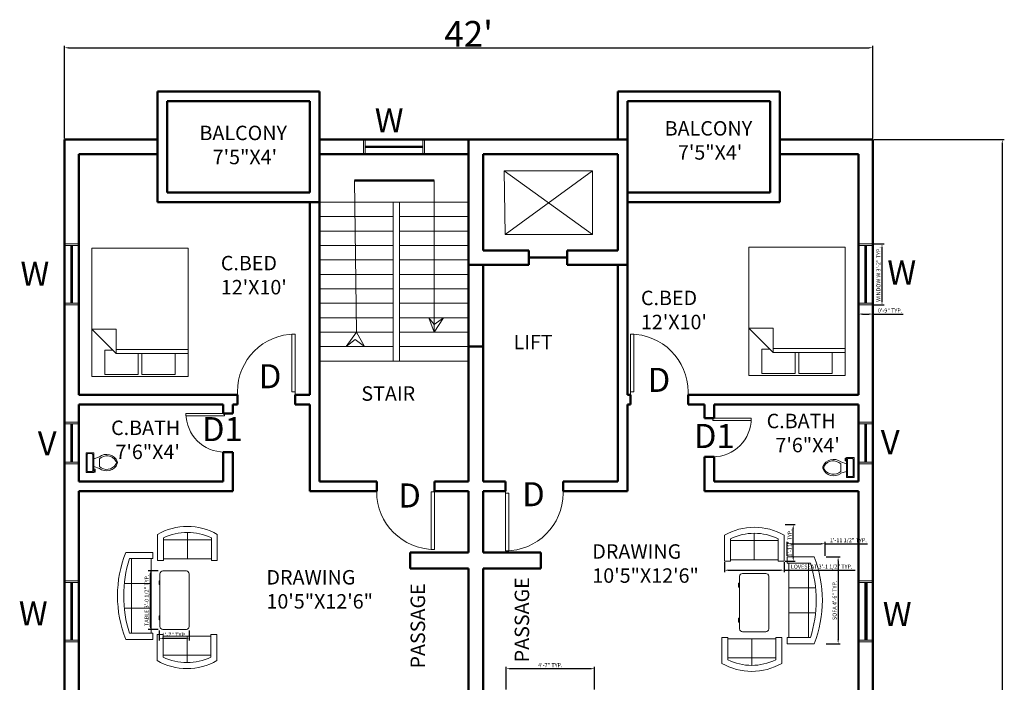
# Model space of a CAD drawing. Units: inches. Extents: x -7040 to -4088, y 6092 to 7645.
# Tile 11 of 11: x -4702 to -4088, y 7176 to 7588. Entities that reach past the tile are written whole.
import ezdxf

# ---------------------------------------------------------------- set-up
doc = ezdxf.new("R2010")
doc.units = ezdxf.units.IN
for name, color, linetype, lineweight in [('A-ANNO-DIMS', 2, 'Continuous', 18), ('A-ANNO-TEXT', 7, 'Continuous', 25), ('A-AREA-IDEN', 3, 'Continuous', 25), ('A-DOOR', 3, 'Continuous', 18), ('A-EQPM', 8, 'Continuous', 18), ('A-FLOR-FIXT', 9, 'Continuous', 13), ('A-FLOR-STRS', 2, 'Continuous', 18), ('A-FURN', 8, 'Continuous', 13), ('A-GLAZ', 4, 'Continuous', 18), ('A-WALL', 7, 'Continuous', 50)]:
    doc.layers.add(name, color=color, linetype=linetype, lineweight=lineweight)
doc.styles.get("Standard").update_dxf_attribs({"font": 'arial.ttf'})
doc.dimstyles.new('ISO-25', dxfattribs={"dimtxt": 2.5, "dimasz": 2.5, "dimexe": 1.25, "dimexo": 0.625, "dimtad": 1, "dimdec": 0, "dimlunit": 3, "dimtxsty": 'Standard', "dimcen": 2.5, "dimadec": 0, "dimazin": 0, "dimtfac": 1, "dimtdec": 0, "dimtmove": 0, "dimatfit": 3, "dimfxl": 1, "dimarcsym": 0})

# ---------------------------------------------------------------- blocks, each defined once
blk = doc.blocks.new('*U8')
for p, q in [((0, 0), (0, -100)), ((750, 0), (750, -100))]:
    blk.add_line(p, q)
blk.add_lwpolyline([(0, 0), (0, 750), (43.75, 750), (43.75, 0)], close=True)
blk.add_arc((0, 0), 750, 0, 90)
blk = doc.blocks.new('Bed - Queen')
for p, q in [((0, -80.00003), (0, 0)), ((0, 0), (59.99999, 0)), ((59.99999, 0), (59.99999, -80.00003)), ((7.99999, -1.2), (28.79998, -1.2)), ((7.99999, -14.4), (7.99999, -1.2)), ((28.79998, -1.2), (28.79998, -14.4)), ((31.19999, -1.2), (51.99999, -1.2)), ((31.19999, -14.4), (31.19999, -1.2)), ((51.99999, -1.2), (51.99999, -16.4)), ((0, -14.4), (44.8, -14.4)), ((44.8, -16.8), (0, -16.8)), ((59.99999, -29.6), (44.8, -14.4)), ((44.8, -14.4), (44.8, -29.6)), ((51.99999, -16.4), (46.79936, -16.4)), ((44.8, -29.6), (59.99999, -29.6)), ((59.99999, -80.00003), (0, -80.00003))]:
    blk.add_line(p, q)
blk = doc.blocks.new('Toilet - top')
for p, q in [((-10, -8.5), (-8, -8.5)), ((-10, -9.5), (-10, -8.5)), ((-7, -9.5), (-10, -9.5)), ((-8, -8.5), (-8, -8)), ((-7, -8), (-7, -9.5)), ((-4, -8), (-6, -14)), ((4, -8), (6, -14)), ((9.5, -6), (9.5, -2)), ((4, -14), (-4, -14))]:
    blk.add_line(p, q)
blk.add_lwpolyline([(10.5, -8), (10.5, 0), (-10.5, 0), (-10.5, -8)], close=True)
for points in [[(-9.5, -2), (-9.5, -6)], [(8.5, -1), (-8.5, -1)], [(-8.5, -7), (8.5, -7)]]:
    blk.add_lwpolyline(points)
for centre, radius, start, end in [((-8.6, -1.9), 0.884, 81.8699, 188.1301), ((-8.6, -6.1), 0.884, 171.8699, 278.1301), ((8.6, -1.9), 0.884, 351.8699, 98.1301), ((8.6, -6.1), 0.884, 261.8699, 8.1301), ((3.5, -21.6), 12.2, 141.4691, 247.9714), ((4.2, -21.8), 11.3, 136.3677, 238.9468), ((-3.5, -21.6), 12.2, 292.0284, 38.5307), ((-4.2, -21.8), 11.3, 301.053, 43.6321), ((0, -27.9), 4, 245.7318, 294.2682), ((0, -29), 4, 254.8605, 285.1395)]:
    blk.add_arc(centre, radius, start, end)
blk = doc.blocks.new('Desk - 30 x 60 in.')
for p, q in [((-26.999995, 0), (26.999995, 0)), ((-29.999995, -27), (-29.999995, -3)), ((29.999995, -3), (29.999995, -27)), ((26.999995, -30), (-26.999995, -30)), ((-20.000005, -30), (-20.000005, -31)), ((-16.000005, -31), (-16.000005, -30)), ((15.999995, -31), (15.999995, -30)), ((19.999995, -30), (19.999995, -31)), ((-20.000005, -31), (-16.000005, -31)), ((19.999995, -31), (15.999995, -31))]:
    blk.add_line(p, q)
for centre, start, end in [((-26.499995, -3.5), 98.1301, 171.8699), ((26.499995, -3.5), 8.130102, 81.8699), ((-26.499995, -26.5), 188.1301, 261.8699), ((26.499995, -26.5), 278.1301, 351.8699)]:
    blk.add_arc(centre, 3.535534, start, end)
blk = doc.blocks.new('Sofa - Roundback 7 ft.')
for p, q in [((-12.00002, -32.4421), (-12.00003, -6.5971)), ((11.99997, -32.4421), (11.99998, -6.5971)), ((-36.000027, -34), (-36.000027, -11.4696)), ((-35.999844, -13.3819), (35.9998, -13.3819)), ((35.99998, -34), (35.99998, -11.4696)), ((-36.000027, -32.4421), (35.99998, -32.4421))]:
    blk.add_line(p, q)
for points in [[(-36.000027, -34), (-42.000027, -34), (-42.000027, -8)], [(41.99998, -8), (41.99998, -34), (35.99998, -34)]]:
    blk.add_lwpolyline(points)
for centre, radius, start, end in [((0, -114.25), 114.25, 68.43141, 111.5686), ((-0.00001, -127.1968), 121.1968, 72.72033, 107.2797)]:
    blk.add_arc(centre, radius, start, end)
blk = doc.blocks.new('Sofa - Roundback Loveseat 5 ft.')
for p, q in [((0, -32.44198), (0, -5.99998)), ((-24, -33.99998), (-24, -11.46958)), ((-23.9998, -13.38178), (23.99986, -13.38178)), ((24.00004, -33.99998), (24.00004, -11.46958)), ((-24, -32.44198), (24.00004, -32.44198))]:
    blk.add_line(p, q)
for points in [[(-24, -33.99998), (-30, -33.99998), (-30, -7.99998)], [(30.00004, -7.99998), (30.00004, -33.99998), (24.00004, -33.99998)]]:
    blk.add_lwpolyline(points)
for centre, radius, start, end in [((0, -60.24998), 60.24998, 60.13715, 119.8628), ((0, -61.38438), 55.38444, 64.32083, 115.6792)]:
    blk.add_arc(centre, radius, start, end)
blk = doc.blocks.new('*D108')
at = {"layer": 'A-ANNO-DIMS', "color": 0, "lineweight": -2, "transparency": 16777216}
for p, q in [((-4673.77, 7514.38), (-4673.77, 7572.26)), ((-4671.27, 7571.01), (-4172.27, 7571.01)), ((-4169.77, 7514.38), (-4169.77, 7572.26))]:
    blk.add_line(p, q, dxfattribs=at)
at = {"layer": 'A-ANNO-DIMS', "color": 0, "transparency": 16777216}
for points in [[(-4671.27, 7571.43), (-4671.27, 7570.59), (-4673.77, 7571.01)], [(-4172.27, 7571.43), (-4172.27, 7570.59), (-4169.77, 7571.01)]]:
    blk.add_solid(points, dxfattribs=at)
at = {"layer": 'Defpoints', "color": 0, "transparency": 16777216}
for p in [(-4169.77, 7571.01), (-4673.77, 7513.76), (-4169.77, 7513.76)]:
    blk.add_point(p, dxfattribs=at)
at = {"layer": 'A-ANNO-DIMS', "color": 0, "transparency": 16777216, "insert": (-4421.77, 7579.67), "char_height": 2.5, "attachment_point": 5}
blk.add_mtext("{\\H6.4x;42'}", dxfattribs=at)
blk = doc.blocks.new('*D109')
at = {"layer": 'A-ANNO-DIMS', "color": 0, "lineweight": -2, "transparency": 16777216}
for p, q in [((-4169.15, 7513.76), (-4087.83, 7513.76)), ((-4089.08, 7511.26), (-4089.08, 6766.26)), ((-4169.15, 6763.76), (-4087.83, 6763.76))]:
    blk.add_line(p, q, dxfattribs=at)
at = {"layer": 'A-ANNO-DIMS', "color": 0, "transparency": 16777216}
for points in [[(-4089.49, 7511.26), (-4088.66, 7511.26), (-4089.08, 7513.76)], [(-4089.49, 6766.26), (-4088.66, 6766.26), (-4089.08, 6763.76)]]:
    blk.add_solid(points, dxfattribs=at)
at = {"layer": 'Defpoints', "color": 0, "transparency": 16777216}
for p in [(-4169.77, 7513.76), (-4169.77, 6763.76), (-4089.08, 6763.76)]:
    blk.add_point(p, dxfattribs=at)
at = {"layer": 'A-ANNO-DIMS', "color": 0, "transparency": 16777216, "insert": (-4097.87, 7138.76), "char_height": 2.5, "attachment_point": 5, "rotation": 90}
blk.add_mtext('{\\H6.4x;62\'-6"}', dxfattribs=at)
blk = doc.blocks.new('WIN-36-B')
for p, q in [((0, 38), (9, 38)), ((0, 37), (9, 37)), ((4, 1), (4, 37)), ((4.5, 1), (4.5, 37)), ((5, 1), (5, 37)), ((0, 1), (9, 1)), ((0, 0), (9, 0))]:
    blk.add_line(p, q)
blk = doc.blocks.new('WIN-24-B')
for p, q in [((0, 26), (9, 26)), ((0, 25), (9, 25)), ((4, 1), (4, 25)), ((4.5, 1), (4.5, 25)), ((5, 1), (5, 25)), ((0, 1), (9, 1)), ((0, 0), (9, 0))]:
    blk.add_line(p, q)
blk = doc.blocks.new('*D118')
at = {"layer": 'A-ANNO-DIMS', "color": 0, "lineweight": -2, "transparency": 16777216}
for p, q in [((-4169.15, 7448.76), (-4162.82, 7448.76)), ((-4164.07, 7413.26), (-4164.07, 7446.26)), ((-4169.15, 7410.76), (-4162.82, 7410.76))]:
    blk.add_line(p, q, dxfattribs=at)
at = {"layer": 'A-ANNO-DIMS', "color": 0, "transparency": 16777216}
for points in [[(-4164.49, 7446.26), (-4163.66, 7446.26), (-4164.07, 7448.76)], [(-4164.49, 7413.26), (-4163.66, 7413.26), (-4164.07, 7410.76)]]:
    blk.add_solid(points, dxfattribs=at)
at = {"layer": 'Defpoints', "color": 0, "transparency": 16777216}
for p in [(-4169.77, 7448.76), (-4164.07, 7448.76), (-4169.77, 7410.76)]:
    blk.add_point(p, dxfattribs=at)
at = {"layer": 'A-ANNO-DIMS', "color": 0, "transparency": 16777216, "insert": (-4165.99, 7429.76), "char_height": 2.5, "attachment_point": 5, "rotation": 90}
blk.add_mtext('WINDOW W 3\'-2" TYP.', dxfattribs=at)
blk = doc.blocks.new('*D119')
at = {"layer": 'A-ANNO-DIMS', "color": 0, "lineweight": -2, "transparency": 16777216}
for p, q in [((-4178.77, 7410.13), (-4178.77, 7403.81)), ((-4169.77, 7410.13), (-4169.77, 7403.81)), ((-4176.27, 7405.06), (-4172.27, 7405.06)), ((-4169.77, 7405.06), (-4150.78, 7405.06))]:
    blk.add_line(p, q, dxfattribs=at)
at = {"layer": 'A-ANNO-DIMS', "color": 0, "transparency": 16777216}
for points in [[(-4176.27, 7405.48), (-4176.27, 7404.64), (-4178.77, 7405.06)], [(-4172.27, 7405.48), (-4172.27, 7404.64), (-4169.77, 7405.06)]]:
    blk.add_solid(points, dxfattribs=at)
at = {"layer": 'Defpoints', "color": 0, "transparency": 16777216}
for p in [(-4178.77, 7410.76), (-4169.77, 7410.76), (-4169.77, 7405.06)]:
    blk.add_point(p, dxfattribs=at)
at = {"layer": 'A-ANNO-DIMS', "color": 0, "transparency": 16777216, "insert": (-4159.03, 7406.96), "char_height": 2.5, "attachment_point": 5}
blk.add_mtext('0\'-9" TYP.', dxfattribs=at)
blk = doc.blocks.new('*D136')
at = {"layer": 'A-ANNO-DIMS', "color": 0, "lineweight": -2, "transparency": 16777216}
for p, q in [((-4262.32, 7250.42), (-4262.32, 7244.2)), ((-4225.01, 7250.42), (-4225.01, 7244.2)), ((-4259.82, 7245.45), (-4227.51, 7245.45)), ((-4225.01, 7245.45), (-4180.89, 7245.45))]:
    blk.add_line(p, q, dxfattribs=at)
at = {"layer": 'A-ANNO-DIMS', "color": 0, "transparency": 16777216}
for points in [[(-4259.82, 7245.87), (-4259.82, 7245.03), (-4262.32, 7245.45)], [(-4227.51, 7245.87), (-4227.51, 7245.03), (-4225.01, 7245.45)]]:
    blk.add_solid(points, dxfattribs=at)
at = {"layer": 'Defpoints', "color": 0, "transparency": 16777216}
for p in [(-4262.32, 7251.05), (-4225.01, 7251.05), (-4225.01, 7245.45)]:
    blk.add_point(p, dxfattribs=at)
at = {"layer": 'A-ANNO-DIMS', "color": 0, "transparency": 16777216, "insert": (-4201.7, 7247.37), "char_height": 2.5, "attachment_point": 5}
blk.add_mtext('LOVESEAT 3\'-1 1/2" TYP.', dxfattribs=at)
blk = doc.blocks.new('*D137')
at = {"layer": 'A-ANNO-DIMS', "color": 0, "lineweight": -2, "transparency": 16777216}
for p, q in [((-4224.38, 7273.85), (-4218.16, 7273.85)), ((-4219.41, 7253.55), (-4219.41, 7271.35)), ((-4224.38, 7251.05), (-4218.16, 7251.05))]:
    blk.add_line(p, q, dxfattribs=at)
at = {"layer": 'A-ANNO-DIMS', "color": 0, "transparency": 16777216}
for points in [[(-4219.83, 7271.35), (-4218.99, 7271.35), (-4219.41, 7273.85)], [(-4219.83, 7253.55), (-4218.99, 7253.55), (-4219.41, 7251.05)]]:
    blk.add_solid(points, dxfattribs=at)
at = {"layer": 'Defpoints', "color": 0, "transparency": 16777216}
for p in [(-4225.01, 7273.85), (-4219.41, 7273.85), (-4225.01, 7251.05)]:
    blk.add_point(p, dxfattribs=at)
at = {"layer": 'A-ANNO-DIMS', "color": 0, "transparency": 16777216, "insert": (-4221.29, 7262.45), "char_height": 2.5, "attachment_point": 5, "rotation": 90}
blk.add_mtext('1\'-11" TYP.', dxfattribs=at)
blk = doc.blocks.new('*D140')
at = {"layer": 'A-ANNO-DIMS', "color": 0, "lineweight": -2, "transparency": 16777216}
for p, q in [((-4198.91, 7253.79), (-4190.15, 7253.79)), ((-4191.4, 7251.29), (-4191.4, 7202.07)), ((-4198.91, 7199.57), (-4190.15, 7199.57))]:
    blk.add_line(p, q, dxfattribs=at)
at = {"layer": 'A-ANNO-DIMS', "color": 0, "transparency": 16777216}
for points in [[(-4191.82, 7251.29), (-4190.98, 7251.29), (-4191.4, 7253.79)], [(-4191.82, 7202.07), (-4190.98, 7202.07), (-4191.4, 7199.57)]]:
    blk.add_solid(points, dxfattribs=at)
at = {"layer": 'Defpoints', "color": 0, "transparency": 16777216}
for p in [(-4199.53, 7253.79), (-4199.53, 7199.57), (-4191.4, 7199.57)]:
    blk.add_point(p, dxfattribs=at)
at = {"layer": 'A-ANNO-DIMS', "color": 0, "transparency": 16777216, "insert": (-4193.32, 7226.68), "char_height": 2.5, "attachment_point": 5, "rotation": 90}
blk.add_mtext('SOFA 4\'-6" TYP.', dxfattribs=at)
blk = doc.blocks.new('*D141')
at = {"layer": 'A-ANNO-DIMS', "color": 0, "lineweight": -2, "transparency": 16777216}
for p, q in [((-4223.2, 7254.42), (-4223.2, 7263.18)), ((-4220.7, 7261.93), (-4202.03, 7261.93)), ((-4199.53, 7254.42), (-4199.53, 7263.18)), ((-4199.53, 7261.93), (-4173.01, 7261.93))]:
    blk.add_line(p, q, dxfattribs=at)
at = {"layer": 'A-ANNO-DIMS', "color": 0, "transparency": 16777216}
for points in [[(-4220.7, 7262.34), (-4220.7, 7261.51), (-4223.2, 7261.93)], [(-4202.03, 7262.34), (-4202.03, 7261.51), (-4199.53, 7261.93)]]:
    blk.add_solid(points, dxfattribs=at)
at = {"layer": 'Defpoints', "color": 0, "transparency": 16777216}
for p in [(-4199.53, 7261.93), (-4223.2, 7253.79), (-4199.53, 7253.79)]:
    blk.add_point(p, dxfattribs=at)
at = {"layer": 'A-ANNO-DIMS', "color": 0, "transparency": 16777216, "insert": (-4185.02, 7263.84), "char_height": 2.5, "attachment_point": 5}
blk.add_mtext('1\'-11 1/2" TYP.', dxfattribs=at)
blk = doc.blocks.new('*D147')
at = {"layer": 'A-ANNO-DIMS', "color": 0, "lineweight": -2, "transparency": 16777216}
for p, q in [((-4398.34, 7171.05), (-4398.34, 7185.33)), ((-4345.84, 7184.08), (-4395.84, 7184.08)), ((-4343.34, 7171.05), (-4343.34, 7185.33))]:
    blk.add_line(p, q, dxfattribs=at)
at = {"layer": 'A-ANNO-DIMS', "color": 0, "transparency": 16777216}
for points in [[(-4395.84, 7184.49), (-4395.84, 7183.66), (-4398.34, 7184.08)], [(-4345.84, 7184.49), (-4345.84, 7183.66), (-4343.34, 7184.08)]]:
    blk.add_solid(points, dxfattribs=at)
at = {"layer": 'Defpoints', "color": 0, "transparency": 16777216}
for p in [(-4398.34, 7184.08), (-4398.34, 7170.43), (-4343.34, 7170.43)]:
    blk.add_point(p, dxfattribs=at)
at = {"layer": 'A-ANNO-DIMS', "color": 0, "transparency": 16777216, "insert": (-4370.84, 7185.95), "char_height": 2.5, "attachment_point": 5}
blk.add_mtext('4\'-7" TYP.', dxfattribs=at)
blk = doc.blocks.new('*D162')
at = {"layer": 'A-ANNO-DIMS', "color": 0, "lineweight": -2, "transparency": 16777216}
for p, q in [((-4615.4, 7244.97), (-4621.5, 7244.97)), ((-4620.25, 7242.47), (-4620.25, 7210.98)), ((-4615.4, 7208.48), (-4621.5, 7208.48))]:
    blk.add_line(p, q, dxfattribs=at)
at = {"layer": 'A-ANNO-DIMS', "color": 0, "transparency": 16777216}
for points in [[(-4620.67, 7242.47), (-4619.83, 7242.47), (-4620.25, 7244.97)], [(-4620.67, 7210.98), (-4619.83, 7210.98), (-4620.25, 7208.48)]]:
    blk.add_solid(points, dxfattribs=at)
at = {"layer": 'Defpoints', "color": 0, "transparency": 16777216}
for p in [(-4614.78, 7244.97), (-4620.25, 7208.48), (-4614.78, 7208.48)]:
    blk.add_point(p, dxfattribs=at)
at = {"layer": 'A-ANNO-DIMS', "color": 0, "transparency": 16777216, "insert": (-4622.17, 7226.73), "char_height": 2.5, "attachment_point": 5, "rotation": 90}
blk.add_mtext('TABLE 3\'-0 1/2" TYP.', dxfattribs=at)
blk = doc.blocks.new('*D163')
at = {"layer": 'A-ANNO-DIMS', "color": 0, "lineweight": -2, "transparency": 16777216}
for p, q in [((-4614.78, 7207.85), (-4614.78, 7201.75)), ((-4595.92, 7207.85), (-4595.92, 7201.75)), ((-4612.28, 7203), (-4598.42, 7203))]:
    blk.add_line(p, q, dxfattribs=at)
at = {"layer": 'A-ANNO-DIMS', "color": 0, "transparency": 16777216}
for points in [[(-4612.28, 7203.42), (-4612.28, 7202.59), (-4614.78, 7203)], [(-4598.42, 7203.42), (-4598.42, 7202.59), (-4595.92, 7203)]]:
    blk.add_solid(points, dxfattribs=at)
at = {"layer": 'Defpoints', "color": 0, "transparency": 16777216}
for p in [(-4614.78, 7208.48), (-4595.92, 7208.48), (-4595.92, 7203)]:
    blk.add_point(p, dxfattribs=at)
at = {"layer": 'A-ANNO-DIMS', "color": 0, "transparency": 16777216, "insert": (-4605.35, 7204.88), "char_height": 2.5, "attachment_point": 5}
blk.add_mtext('1\'-7" TYP.', dxfattribs=at)

msp = doc.modelspace()

# ---------------------------------------------------------------- linework, layer by layer
at = {"layer": 'A-EQPM'}
for p, q in [((-4399.56, 7494.25), (-4344.57, 7494.25)), ((-4399.04, 7454.68), (-4399.56, 7494.25)), ((-4399.56, 7494.25), (-4344.57, 7454.68)), ((-4344.57, 7494.25), (-4399.04, 7454.68)), ((-4344.57, 7494.25), (-4344.57, 7454.68)), ((-4344.57, 7454.68), (-4399.04, 7454.68))]:
    msp.add_line(p, q, dxfattribs=at)
at = {"layer": 'A-FLOR-STRS'}
for p, q in [((-4492.85, 7488.24), (-4491.77, 7393.76)), ((-4443.27, 7393.76), (-4443.27, 7488.24)), ((-4514.77, 7474.76), (-4421.77, 7474.76)), ((-4468.77, 7375.76), (-4468.77, 7474.76)), ((-4464.77, 7375.76), (-4464.77, 7474.76)), ((-4514.77, 7465.76), (-4468.77, 7465.76)), ((-4464.77, 7465.76), (-4421.77, 7465.76)), ((-4514.77, 7456.76), (-4468.77, 7456.76)), ((-4464.77, 7456.76), (-4421.77, 7456.76)), ((-4514.77, 7447.76), (-4468.77, 7447.76)), ((-4464.77, 7447.76), (-4421.77, 7447.76)), ((-4514.77, 7438.76), (-4468.77, 7438.76)), ((-4464.77, 7438.76), (-4421.77, 7438.76)), ((-4514.77, 7429.76), (-4468.77, 7429.76)), ((-4464.77, 7429.76), (-4421.77, 7429.76)), ((-4514.77, 7420.76), (-4468.77, 7420.76)), ((-4464.77, 7420.76), (-4421.77, 7420.76)), ((-4514.77, 7411.76), (-4468.77, 7411.76)), ((-4464.77, 7411.76), (-4421.77, 7411.76)), ((-4514.77, 7402.76), (-4468.77, 7402.76)), ((-4464.77, 7402.76), (-4421.77, 7402.76)), ((-4443.27, 7398.63), (-4446.58, 7402.76)), ((-4446.58, 7402.76), (-4443.27, 7393.76)), ((-4443.27, 7393.76), (-4437.33, 7402.76)), ((-4437.33, 7402.76), (-4443.27, 7398.63)), ((-4514.77, 7393.76), (-4468.77, 7393.76)), ((-4491.77, 7393.76), (-4498.16, 7384.76)), ((-4486.75, 7384.76), (-4491.77, 7393.76)), ((-4464.77, 7393.76), (-4421.77, 7393.76)), ((-4514.77, 7384.76), (-4468.77, 7384.76)), ((-4501.85, 7384.76), (-4491.73, 7384.76)), ((-4498.16, 7384.76), (-4492.45, 7389.13)), ((-4492.45, 7389.13), (-4486.75, 7384.76)), ((-4491.73, 7384.76), (-4483.48, 7384.76)), ((-4464.77, 7384.76), (-4421.77, 7384.76)), ((-4514.77, 7375.76), (-4421.77, 7375.76))]:
    msp.add_line(p, q, dxfattribs=at)
at = {"layer": 'A-GLAZ'}
for p, q in [((-4178.77, 7238.76), (-4169.77, 7238.76)), ((-4178.77, 7237.76), (-4169.77, 7237.76)), ((-4174.77, 7201.76), (-4174.77, 7237.76)), ((-4174.27, 7201.76), (-4174.27, 7237.76)), ((-4178.77, 7201.76), (-4169.77, 7201.76)), ((-4178.77, 7200.76), (-4169.77, 7200.76))]:
    msp.add_line(p, q, dxfattribs=at)
at = {"layer": 'A-WALL'}
for p, q in [((-4615.77, 7543.76), (-4514.77, 7543.76)), ((-4615.77, 7474.76), (-4615.77, 7543.76)), ((-4514.77, 7300.76), (-4514.77, 7543.76)), ((-4328.77, 7543.76), (-4328.77, 7513.76)), ((-4328.77, 7543.76), (-4227.77, 7543.76)), ((-4227.77, 7543.76), (-4227.77, 7474.76)), ((-4609.77, 7537.76), (-4520.77, 7537.76)), ((-4609.77, 7480.76), (-4609.77, 7537.76)), ((-4520.77, 7480.76), (-4520.77, 7537.76)), ((-4322.77, 7537.76), (-4322.77, 7474.76)), ((-4322.77, 7537.76), (-4233.77, 7537.76)), ((-4233.77, 7537.76), (-4233.77, 7480.76)), ((-4673.77, 7513.76), (-4615.77, 7513.76)), ((-4673.77, 6763.76), (-4673.77, 7513.76)), ((-4514.77, 7513.76), (-4322.77, 7513.76)), ((-4421.77, 7513.76), (-4421.77, 7300.76)), ((-4227.77, 7513.76), (-4169.77, 7513.76)), ((-4169.77, 7513.76), (-4169.77, 6763.76)), ((-4664.77, 7504.76), (-4615.77, 7504.76)), ((-4664.77, 7354.76), (-4664.77, 7504.76)), ((-4514.77, 7504.76), (-4421.77, 7504.76)), ((-4412.77, 7504.76), (-4412.77, 7444.76)), ((-4412.77, 7504.76), (-4328.77, 7504.76)), ((-4328.77, 7504.76), (-4328.77, 7444.76)), ((-4227.77, 7504.76), (-4178.77, 7504.76)), ((-4178.77, 7504.76), (-4178.77, 7354.76)), ((-4443.27, 7488.24), (-4492.85, 7488.24)), ((-4609.77, 7480.76), (-4520.77, 7480.76)), ((-4322.77, 7480.76), (-4233.77, 7480.76)), ((-4615.77, 7474.76), (-4514.77, 7474.76)), ((-4520.77, 7354.76), (-4520.77, 7474.76)), ((-4322.77, 7474.76), (-4227.77, 7474.76)), ((-4322.77, 7474.76), (-4322.77, 7354.76)), ((-4412.77, 7444.76), (-4384.21, 7444.76)), ((-4384.21, 7444.76), (-4384.21, 7435.76)), ((-4384.21, 7440.26), (-4360.25, 7440.26)), ((-4360.25, 7444.76), (-4360.25, 7435.76)), ((-4360.25, 7444.76), (-4328.77, 7444.76)), ((-4421.77, 7435.76), (-4384.21, 7435.76)), ((-4412.77, 7435.76), (-4412.77, 7300.76)), ((-4360.25, 7435.76), (-4322.77, 7435.76)), ((-4328.77, 7435.76), (-4328.77, 7300.76)), ((-4421.77, 7384.76), (-4412.77, 7384.76)), ((-4664.77, 7354.76), (-4565.93, 7354.76)), ((-4565.93, 7354.76), (-4565.93, 7348.76)), ((-4529.93, 7354.76), (-4529.93, 7348.76)), ((-4529.93, 7354.76), (-4520.77, 7354.76)), ((-4322.77, 7354.76), (-4320.95, 7354.76)), ((-4320.95, 7354.76), (-4320.95, 7348.76)), ((-4284.95, 7354.76), (-4284.95, 7348.76)), ((-4284.95, 7354.76), (-4178.77, 7354.76)), ((-4664.77, 7348.76), (-4574.77, 7348.76)), ((-4664.77, 7300.76), (-4664.77, 7348.76)), ((-4574.77, 7343.08), (-4574.77, 7348.76)), ((-4568.77, 7348.76), (-4565.93, 7348.76)), ((-4568.77, 7343.08), (-4568.77, 7348.76)), ((-4529.93, 7348.76), (-4520.77, 7348.76)), ((-4520.77, 7294.76), (-4520.77, 7348.76)), ((-4322.77, 7348.76), (-4320.95, 7348.76)), ((-4322.77, 7348.76), (-4322.77, 7294.76)), ((-4284.95, 7348.76), (-4274.77, 7348.76)), ((-4274.77, 7348.76), (-4274.77, 7340.09)), ((-4268.77, 7348.76), (-4268.77, 7340.09)), ((-4268.77, 7348.76), (-4178.77, 7348.76)), ((-4178.77, 7348.76), (-4178.77, 7300.76)), ((-4574.77, 7343.08), (-4568.77, 7343.08)), ((-4274.77, 7340.09), (-4268.77, 7340.09)), ((-4574.77, 7300.76), (-4574.77, 7319.08)), ((-4574.77, 7319.08), (-4568.77, 7319.08)), ((-4568.77, 7294.76), (-4568.77, 7319.08)), ((-4274.77, 7316.09), (-4268.77, 7316.09)), ((-4274.77, 7316.09), (-4274.77, 7294.76)), ((-4268.77, 7316.09), (-4268.77, 7300.76)), ((-4664.77, 7300.76), (-4574.77, 7300.76)), ((-4514.77, 7300.76), (-4479.09, 7300.76)), ((-4479.09, 7300.76), (-4479.09, 7294.76)), ((-4443.09, 7300.76), (-4443.09, 7294.76)), ((-4443.09, 7300.76), (-4421.77, 7300.76)), ((-4412.77, 7300.76), (-4398.86, 7300.76)), ((-4398.86, 7300.76), (-4398.86, 7294.76)), ((-4362.86, 7300.76), (-4362.86, 7294.76)), ((-4362.86, 7300.76), (-4328.77, 7300.76)), ((-4268.77, 7300.76), (-4178.77, 7300.76)), ((-4664.77, 7294.76), (-4568.77, 7294.76)), ((-4664.77, 7144.76), (-4664.77, 7294.76)), ((-4520.77, 7294.76), (-4479.09, 7294.76)), ((-4443.09, 7294.76), (-4421.77, 7294.76)), ((-4421.77, 7294.76), (-4421.77, 7256.45)), ((-4412.77, 7294.76), (-4412.77, 7256.45)), ((-4412.77, 7294.76), (-4398.86, 7294.76)), ((-4362.86, 7294.76), (-4328.77, 7294.76)), ((-4328.77, 7294.76), (-4322.77, 7294.76)), ((-4274.77, 7294.76), (-4178.77, 7294.76)), ((-4178.77, 7294.76), (-4178.77, 7144.76)), ((-4421.77, 7256.45), (-4458.21, 7256.45)), ((-4458.21, 7256.45), (-4458.21, 7246.46)), ((-4412.77, 7256.45), (-4376.73, 7256.45)), ((-4376.73, 7256.45), (-4376.73, 7246.46)), ((-4458.21, 7246.46), (-4421.77, 7246.46)), ((-4421.77, 7246.46), (-4421.77, 7052.76)), ((-4376.73, 7246.46), (-4412.77, 7246.46)), ((-4412.77, 7246.46), (-4412.77, 7052.76)), ((-4173.77, 7201.76), (-4173.77, 7237.76))]:
    msp.add_line(p, q, dxfattribs=at)

# ---------------------------------------------------------------- block references
at = {"layer": 'A-DOOR'}
for p, xscale, yscale, zscale in [((-4529.93, 7356.56), -0.0479999999999998, 0.0479999999999998, 0.0479999999999998), ((-4320.95, 7356.56), 0.0479999999999999, 0.0479999999999999, 0.0479999999999999)]:
    msp.add_blockref('*U8', p, dxfattribs=dict(at, xscale=xscale, yscale=yscale, zscale=zscale))
for p, xscale, yscale, zscale, rotation in [((-4573.97, 7343.06), -0.0319901519123588, 0.0319901519123588, 0.0319901519123588, 90), ((-4269.53, 7340.11), 0.0319999999999999, 0.0319999999999999, 0.0319999999999999, 270), ((-4443.09, 7294.36), 0.0479999999999998, 0.0479999999999998, 0.0479999999999998, 180), ((-4398.86, 7293.44), -0.0479266341713571, 0.0479266341713571, 0.0479266341713571, 180)]:
    msp.add_blockref('*U8', p, dxfattribs=dict(at, xscale=xscale, yscale=yscale, zscale=zscale, rotation=rotation))
at = {"layer": 'A-FLOR-FIXT', "xscale": 0.5917696287157074, "yscale": 0.5917696287157074, "zscale": 0.5917696287157074}
for p, rotation in [((-4660.25, 7312.48), 90), ((-4181.5, 7309.39), 270)]:
    msp.add_blockref('Toilet - top', p, dxfattribs=dict(at, rotation=rotation))
at = {"layer": 'A-FURN', "rotation": 180}
for p in [(-4596.63, 7366.15), (-4187.07, 7366.77)]:
    msp.add_blockref('Bed - Queen', p, dxfattribs=at)
at = {"layer": 'A-FURN', "xscale": 0.6218676739411199, "yscale": 0.6218676739411199, "zscale": 0.6218676739411199}
for p in [(-4597.08, 7272.72), (-4243.66, 7272.19)]:
    msp.add_blockref('Sofa - Roundback Loveseat 5 ft.', p, dxfattribs=at)
at = {"layer": 'A-FURN'}
for name, p, xscale, yscale, zscale, rotation in [('Sofa - Roundback 7 ft.', (-4640.67, 7229.46), 0.645508341035607, 0.645508341035607, 0.645508341035607, 89.99999999999999), ('Sofa - Roundback 7 ft.', (-4201.26, 7226.68), 0.645508341035607, 0.645508341035607, 0.645508341035607, 270), ('Desk - 30 x 60 in.', (-4595.92, 7226.73), 0.6082896353213999, 0.6082896353213999, 0.6082896353213999, 270), ('Desk - 30 x 60 in.', (-4234.66, 7225.24), 0.6082896353213999, 0.6082896353213999, 0.6082896353213999, 270), ('Sofa - Roundback Loveseat 5 ft.', (-4597.31, 7184.16), 0.6218676739411199, 0.6218676739411199, 0.6218676739411199, 180), ('Sofa - Roundback Loveseat 5 ft.', (-4245.25, 7182.43), 0.6218676739411199, 0.6218676739411199, 0.6218676739411199, 180)]:
    msp.add_blockref(name, p, dxfattribs=dict(at, xscale=xscale, yscale=yscale, zscale=zscale, rotation=rotation))
at = {"layer": 'A-GLAZ', "rotation": 269.9999999999954}
msp.add_blockref('WIN-36-B', (-4487.27, 7513.76), dxfattribs=at)
at = {"layer": 'A-GLAZ'}
for name, p in [('WIN-36-B', (-4673.77, 7410.76)), ('WIN-36-B', (-4178.77, 7410.76)), ('WIN-24-B', (-4673.77, 7311.76)), ('WIN-24-B', (-4178.77, 7311.76)), ('WIN-36-B', (-4673.77, 7200.76))]:
    msp.add_blockref(name, p, dxfattribs=at)

# ---------------------------------------------------------------- texts
at = {"layer": 'A-ANNO-TEXT', "char_height": 15, "attachment_point": 1}
for s, insert in [('{W}', (-4480.3, 7533.34)), ('{W}', (-4701.16, 7437.67)), ('{W}', (-4160.74, 7438.45)), ('{D}', (-4552.56, 7373.81)), ('{D}', (-4310.15, 7371.55)), ('{D1}', (-4588, 7340.87)), ('{D1}', (-4281.33, 7336.58)), ('{V}', (-4690.37, 7332.04)), ('{V}', (-4164.86, 7332.75)), ('{D}', (-4465.61, 7299.51)), ('{D}', (-4388.38, 7300.31)), ('{W}', (-4702.16, 7226.04)), ('{W}', (-4163.56, 7225.66))]:
    msp.add_mtext_dynamic_manual_height_columns(s, width=939.647, gutter_width=12.5, heights=[0], dxfattribs=dict(at, insert=insert))
at = {"layer": 'A-AREA-IDEN', "char_height": 9, "attachment_point": 1}
for s, insert in [('{BALCONY\\P   7\'5"X4\'}', (-4299.54, 7525.29)), ('{BALCONY\\P   7\'5"X4\'}', (-4589.56, 7522.43)), ("{ C.BED\\P 12'X10'}", (-4578.99, 7441.32)), ("{ C.BED\\P 12'X10'}", (-4317.09, 7419.62)), ('{LIFT}', (-4393.77, 7392.12)), ('{STAIR}', (-4488.63, 7360.04)), ('{ C.BATH\\P   7\'6"X4\'}', (-4238.73, 7342.93)), ('{  C.BATH\\P   7\'6"X4\'}', (-4650.16, 7338.69)), ('{ DRAWING\\P 10\'5"X12\'6"}', (-4347.4, 7261.61)), ('{ DRAWING\\P 10\'5"X12\'6"}', (-4550.54, 7245.54))]:
    msp.add_mtext_dynamic_manual_height_columns(s, width=1007.2961, gutter_width=12.5, heights=[0], dxfattribs=dict(at, insert=insert))
at = {"layer": 'A-AREA-IDEN', "char_height": 9, "attachment_point": 1, "rotation": 90}
for insert in [(-4393.05, 7188.05), (-4457.94, 7184.21)]:
    msp.add_mtext_dynamic_manual_height_columns('{PASSAGE}', width=1007.2961, gutter_width=12.5, heights=[0], dxfattribs=dict(at, insert=insert))

# ---------------------------------------------------------------- dimensions: what is measured, and where the dimension line sits
at = {"layer": 'A-ANNO-DIMS'}
for base, p1, p2, text, override, picture, middle in [((-4169.77, 7571.01), (-4673.77, 7513.76), (-4169.77, 7513.76), '{\\H6.4x;<>}', {"dimclrd": 0, "dimclre": 0, "dimclrt": 0}, '*D108', (-4421.77, 7579.67)), ((-4169.77, 7405.06), (-4178.77, 7410.76), (-4169.77, 7410.76), '<> TYP.', {"dimdec": 1, "dimrnd": 0, "dimzin": 1, "dimlunit": 4, "dimfrac": 2}, '*D119', (-4159.03, 7406.96)), ((-4199.53, 7261.93), (-4223.2, 7253.79), (-4199.53, 7253.79), '<> TYP.', {"dimdec": 1, "dimrnd": 0, "dimzin": 1, "dimlunit": 4, "dimfrac": 2}, '*D141', (-4185.02, 7263.84)), ((-4225.01, 7245.45), (-4262.32, 7251.05), (-4225.01, 7251.05), 'LOVESEAT <> TYP.', {"dimdec": 1, "dimrnd": 0, "dimzin": 1, "dimlunit": 4, "dimfrac": 2}, '*D136', (-4201.7, 7247.37)), ((-4595.92, 7203), (-4614.78, 7208.48), (-4595.92, 7208.48), '<> TYP.', {"dimdec": 1, "dimrnd": 0, "dimzin": 1, "dimlunit": 4, "dimfrac": 2}, '*D163', (-4605.35, 7204.88))]:
    dim = msp.add_linear_dim(base=base, p1=p1, p2=p2, text=text, dimstyle='ISO-25', override=override, dxfattribs=at)
    dim.commit()
    dim.dimension.update_dxf_attribs({"geometry": picture, "text_midpoint": middle})
for base, p1, p2, angle, text, override, picture, middle in [((-4089.08, 6763.76), (-4169.77, 7513.76), (-4169.77, 6763.76), 90, '{\\H6.4x;<>}', {"dimclrd": 0, "dimclre": 0, "dimclrt": 0}, '*D109', (-4097.87, 7138.76)), ((-4164.07, 7448.76), (-4169.77, 7410.76), (-4169.77, 7448.76), 90, 'WINDOW W <> TYP.', {"dimdec": 1, "dimrnd": 0, "dimzin": 1, "dimlunit": 4, "dimfrac": 2}, '*D118', (-4165.99, 7429.76)), ((-4219.41, 7273.85), (-4225.01, 7251.05), (-4225.01, 7273.85), 90, '<> TYP.', {"dimdec": 1, "dimrnd": 0, "dimzin": 1, "dimlunit": 4, "dimfrac": 2}, '*D137', (-4221.29, 7262.45)), ((-4191.4, 7199.57), (-4199.53, 7253.79), (-4199.53, 7199.57), 270, 'SOFA <> TYP.', {"dimdec": 1, "dimrnd": 0, "dimzin": 1, "dimlunit": 4, "dimfrac": 2}, '*D140', (-4193.32, 7226.68)), ((-4620.25, 7208.48), (-4614.78, 7244.97), (-4614.78, 7208.48), 270, 'TABLE <> TYP.', {"dimdec": 1, "dimrnd": 0, "dimzin": 1, "dimlunit": 4, "dimfrac": 2}, '*D162', (-4622.17, 7226.73)), ((-4398.34, 7184.08), (-4343.34, 7170.43), (-4398.34, 7170.43), 180, '<> TYP.', {"dimdec": 1, "dimrnd": 0, "dimzin": 1, "dimlunit": 4, "dimfrac": 2}, '*D147', (-4370.84, 7185.95))]:
    dim = msp.add_linear_dim(base=base, p1=p1, p2=p2, angle=angle, text=text, dimstyle='ISO-25', override=override, dxfattribs=at)
    dim.commit()
    dim.dimension.update_dxf_attribs({"geometry": picture, "text_midpoint": middle})

doc.saveas('drawing.dxf')
